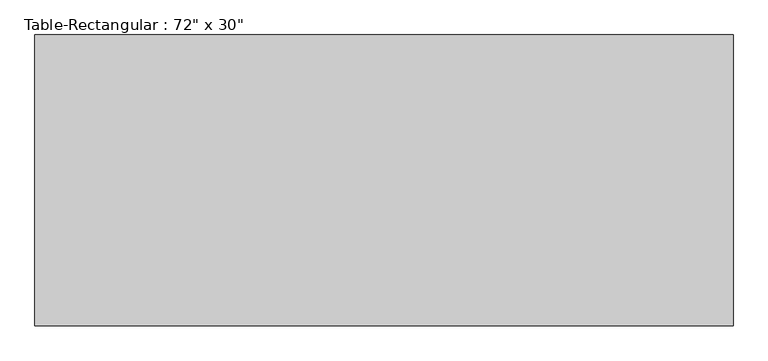
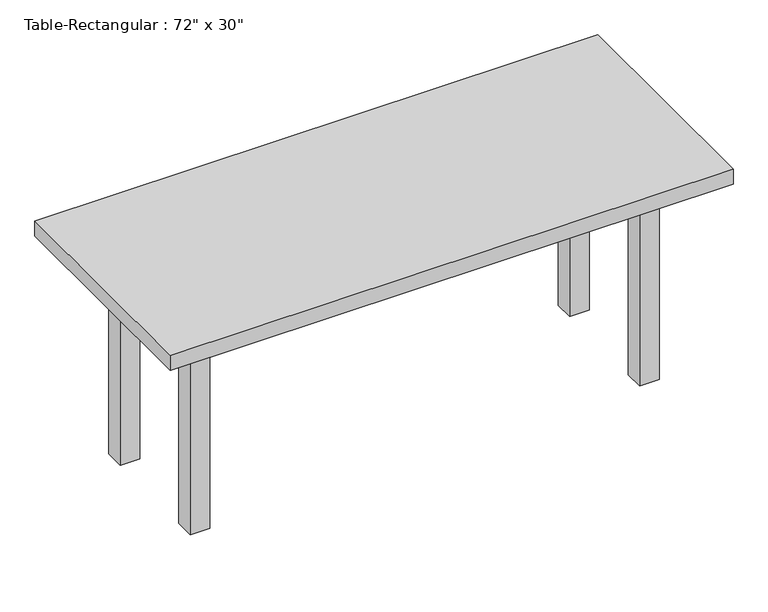
"""IFC4 building model written with IfcOpenShell, lengths in millimetres: furniture geometry."""

from ifc_helpers import new_model, si_unit, frame, origin, origin_with_axes, place, context, project, spatial, polyline, outline, extrude, source, transform, mapped, element, save


def furniture_a5b052b6(model_context):
    return source(origin(), model_context, "Body", "SweptSolid", [
        extrude(outline(polyline([(698.5, 190.5), (698.5, 165.1), (-698.5, 165.1), (-698.5, 190.5), (698.5, 190.5)])), frame((0.0, 0.0, 609.6), z_axis=(0.0, 0.0, 1.0), x_axis=(1.0, 0.0, 0.0)), (0.0, 0.0, 1.0), 101.6),
        extrude(outline(polyline([(698.5, -190.5), (-698.5, -190.5), (-698.5, -165.1), (698.5, -165.1), (698.5, -190.5)])), frame((0.0, 0.0, 609.6), z_axis=(0.0, 0.0, 1.0), x_axis=(1.0, 0.0, 0.0)), (0.0, 0.0, 1.0), 101.6),
        extrude(outline(polyline([(-711.2, -165.1), (-736.6, -165.1), (-736.6, 165.1), (-711.2, 165.1), (-711.2, -165.1)])), frame((0.0, 0.0, 609.6), z_axis=(0.0, 0.0, 1.0), x_axis=(1.0, 0.0, 0.0)), (0.0, 0.0, 1.0), 101.6),
        extrude(outline(polyline([(711.2, -165.1), (711.2, 165.1), (736.6, 165.1), (736.6, -165.1), (711.2, -165.1)])), frame((0.0, 0.0, 609.6), z_axis=(0.0, 0.0, 1.0), x_axis=(1.0, 0.0, 0.0)), (0.0, 0.0, 1.0), 101.6),
        extrude(outline(polyline([(914.4, 381.0), (914.4, -381.0), (-914.4, -381.0), (-914.4, 381.0), (914.4, 381.0)])), frame((0.0, 0.0, 711.2), z_axis=(0.0, 0.0, 1.0), x_axis=(1.0, 0.0, 0.0)), (0.0, 0.0, 1.0), 50.8),
        extrude(outline(polyline([(-698.5, 228.6), (-698.5, 165.1), (-762.0, 165.1), (-762.0, 228.6), (-698.5, 228.6)])), origin_with_axes(), (0.0, 0.0, 1.0), 711.2),
        extrude(outline(polyline([(698.5, 228.6), (762.0, 228.6), (762.0, 165.1), (698.5, 165.1), (698.5, 228.6)])), origin_with_axes(), (0.0, 0.0, 1.0), 711.2),
        extrude(outline(polyline([(-698.5, -228.6), (-762.0, -228.6), (-762.0, -165.1), (-698.5, -165.1), (-698.5, -228.6)])), origin_with_axes(), (0.0, 0.0, 1.0), 711.2),
        extrude(outline(polyline([(698.5, -228.6), (698.5, -165.1), (762.0, -165.1), (762.0, -228.6), (698.5, -228.6)])), origin_with_axes(), (0.0, 0.0, 1.0), 711.2),
    ])


if __name__ == "__main__":
    model = new_model("IFC4")
    model_context = context("Model", 3, world=origin())
    ifc_project = project(units=[si_unit("LENGTHUNIT", "METRE", prefix="MILLI")], contexts=[model_context])
    site = spatial("IfcSite", under=ifc_project)
    building = spatial("IfcBuilding", under=site)
    placement = place(None, origin())
    furniture_shape = furniture_a5b052b6(model_context)
    element("IfcFurniture", 1, ObjectType="Table-Rectangular : 72\" x 30\"", at=placement, inside=building, context=model_context, shape_type="MappedRepresentation", body=[
        mapped(furniture_shape, transform((0.0, 0.0, 0.0), x_axis=(1.0, 0.0, 0.0), y_axis=(0.0, 1.0, 0.0), z_axis=(0.0, 0.0, 1.0))),
    ])
    save(model, "model.ifc")

# Revit data of these elements
# Type "Table-Rectangular : 72\" x 30\""
#   Assembly Code = "E2020200"
#   Height = 2' - 6"
#   Length = 6' - 0"
#   Width = 2' - 6"
#   Base Material = Birch
#   Top Material = Gypsum Wall Board
#   Default Elevation = 0
# Element 1 (IfcFurniture, "Table-Rectangular : 72\" x 30\"")
#   Materials on its faces: "Birch", "Gypsum Wall Board"
# Materials
#   "Birch": class "Wood", colour RGB 224 178 126, transparency 0, Description = "Betula Alleghaniensis", Cost = 0
#   "Gypsum Wall Board": class "Generic", colour RGB 127 127 127, transparency 0, Description = "Gypsum Wall Board", Cost = 0
